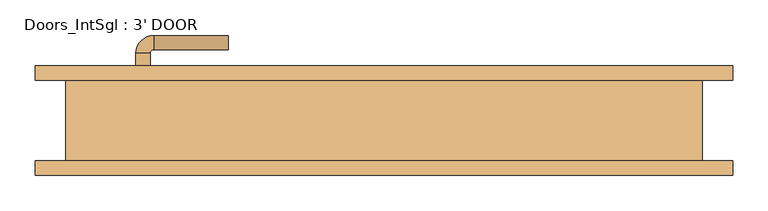
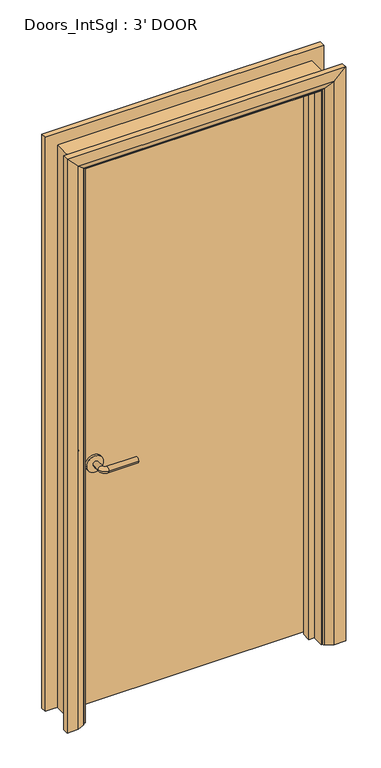
"""IFC4 building model written with IfcOpenShell, lengths in millimetres: door geometry, Doors_IntSgl : 3' DOOR."""

from ifc_helpers import new_model, si_unit, point, frame, frame_2d, origin, place, context, project, spatial, polyline, circle_curve, ellipse_curve, trimmed, segment, composite_curve, outline, extrude, faceted_brep, source, transform, mapped, element, save
from ifc_brep_helpers import plane_surface, cylinder_surface, revolved_surface, advanced_brep


def doors_intsgl_3_door_77e94e6e(model_context):
    return source(origin(), model_context, "Body", "SolidModel", [
        advanced_brep(
        [(-350.2, 11.15, 900.0), (-330.2, 11.15, 900.0), (-330.2, -18.85, 900.0), (-350.2, -18.85, 900.0), (-325.2, -23.85, 900.0), (-325.2, -43.85, 900.0), (-220.2, -43.85, 900.0), (-220.2, -23.85, 900.0)],
        [
            (0, 1, circle_curve(frame((-340.2, 11.15, 900.0), z_axis=(0.0, 1.0, 0.0), x_axis=(1.0, 0.0, 0.0)), 10.0)),
            (1, 0, circle_curve(frame((-340.2, 11.15, 900.0), z_axis=(0.0, 1.0, 0.0), x_axis=(1.0, 0.0, 0.0)), 10.0)),
            (1, 2),
            (2, 3, circle_curve(frame((-340.2, -18.85, 900.0), z_axis=(0.0, 1.0, 0.0), x_axis=(1.0, 0.0, 0.0)), 10.0)),
            (3, 0),
            (3, 2, circle_curve(frame((-340.2, -18.85, 900.0), z_axis=(0.0, 1.0, 0.0), x_axis=(1.0, 0.0, 0.0)), 10.0)),
            (4, 5, circle_curve(frame((-325.2, -33.85, 900.0), z_axis=(-1.0, 0.0, 0.0), x_axis=(0.0, 1.0, 0.0)), 10.0)),
            (5, 3, circle_curve(frame((-325.2, -18.85, 900.0), z_axis=(0.0, 0.0, -1.0), x_axis=(-1.0, 0.0, 0.0)), 25.0)),
            (2, 4, circle_curve(frame((-325.2, -18.85, 900.0), z_axis=(0.0, 0.0, 1.0), x_axis=(-1.0, 0.0, 0.0)), 5.0)),
            (5, 4, circle_curve(frame((-325.2, -33.85, 900.0), z_axis=(-1.0, 0.0, 0.0), x_axis=(0.0, 1.0, 0.0)), 10.0)),
            (6, 7, circle_curve(frame((-220.2, -33.85, 900.0), z_axis=(1.0, 0.0, 0.0), x_axis=(0.0, 1.0, 0.0)), 10.0)),
            (7, 6, circle_curve(frame((-220.2, -33.85, 900.0), z_axis=(1.0, 0.0, 0.0), x_axis=(0.0, 1.0, 0.0)), 10.0)),
            (4, 7),
            (6, 5),
        ],
        [
            plane_surface(frame((-340.2, 11.15, 900.0), z_axis=(0.0, 1.0, 0.0), x_axis=(0.0, 0.0, 1.0))),
            cylinder_surface(frame((-340.2, 11.15, 900.0), z_axis=(0.0, 1.0, 0.0), x_axis=(1.0, 0.0, 0.0)), 10.0),
            revolved_surface(trimmed(ellipse_curve(frame((-340.2, -18.85, 900.0), z_axis=(0.0, -1.0, 0.0), x_axis=(1.0, 0.0, 0.0)), 10.0, 10.0), [point((-350.2, -18.85, 900.0))], [point((-330.2, -18.85, 900.0))], True, "CARTESIAN"), (-325.2, -18.85, 900.0), (0.0, 0.0, -1.0)),
            revolved_surface(trimmed(ellipse_curve(frame((-340.2, -18.85, 900.0), z_axis=(0.0, -1.0, 0.0), x_axis=(1.0, 0.0, 0.0)), 10.0, 10.0), [point((-330.2, -18.85, 900.0))], [point((-350.2, -18.85, 900.0))], True, "CARTESIAN"), (-325.2, -18.85, 900.0), (0.0, 0.0, -1.0)),
            plane_surface(frame((-220.2, -33.85, 900.0), z_axis=(1.0, 0.0, 0.0), x_axis=(0.0, 0.0, 1.0))),
            cylinder_surface(frame((-325.2, -33.85, 900.0), z_axis=(-1.0, 0.0, 0.0), x_axis=(0.0, 1.0, 0.0)), 10.0),
        ],
        [
            (0, [[1, 2]]),
            (1, [[3, 4, 5, -2]]),
            (1, [[-5, 6, -3, -1]]),
            (2, [[7, 8, -4, 9]]),
            (3, [[10, -9, -6, -8]]),
            (4, [[11, 12]]),
            (5, [[13, -11, 14, -7]]),
            (5, [[-14, -12, -13, -10]]),
        ],
    ),
        extrude(outline(composite_curve([segment(trimmed(circle_curve(frame_2d((900.0, -342.7)), 30.0), [point((900.0, -372.7))], [point((900.0, -312.7))], False, "CARTESIAN"), True, "CONTINUOUS"), segment(trimmed(circle_curve(frame_2d((900.0, -342.7)), 30.0), [point((900.0, -312.7))], [point((900.0, -372.7))], False, "CARTESIAN"), True, "CONTINUOUS")], self_intersect=False)), frame((0.0, 11.15, 0.0), z_axis=(0.0, 1.0, 0.0), x_axis=(0.0, 0.0, 1.0)), (0.0, 0.0, 1.0), 8.0),
        advanced_brep(
        [(-350.2, 65.15, 900.0), (-330.2, 65.15, 900.0), (-350.2, 95.15, 900.0), (-330.2, 95.15, 900.0), (-325.2, 100.15, 900.0), (-325.2, 120.15, 900.0), (-220.2, 120.15, 900.0), (-220.2, 100.15, 900.0)],
        [
            (0, 1, circle_curve(frame((-340.2, 65.15, 900.0), z_axis=(0.0, -1.0, 0.0), x_axis=(1.0, 0.0, 0.0)), 10.0)),
            (1, 0, circle_curve(frame((-340.2, 65.15, 900.0), z_axis=(0.0, -1.0, 0.0), x_axis=(1.0, 0.0, 0.0)), 10.0)),
            (0, 2),
            (2, 3, circle_curve(frame((-340.2, 95.15, 900.0), z_axis=(0.0, -1.0, 0.0), x_axis=(1.0, 0.0, 0.0)), 10.0)),
            (3, 1),
            (3, 2, circle_curve(frame((-340.2, 95.15, 900.0), z_axis=(0.0, -1.0, 0.0), x_axis=(1.0, 0.0, 0.0)), 10.0)),
            (4, 3, circle_curve(frame((-325.2, 95.15, 900.0), z_axis=(0.0, 0.0, 1.0), x_axis=(-1.0, 0.0, 0.0)), 5.0)),
            (2, 5, circle_curve(frame((-325.2, 95.15, 900.0), z_axis=(0.0, 0.0, -1.0), x_axis=(-1.0, 0.0, 0.0)), 25.0)),
            (5, 4, circle_curve(frame((-325.2, 110.15, 900.0), z_axis=(-1.0, 0.0, 0.0), x_axis=(0.0, -1.0, 0.0)), 10.0)),
            (4, 5, circle_curve(frame((-325.2, 110.15, 900.0), z_axis=(-1.0, 0.0, 0.0), x_axis=(0.0, -1.0, 0.0)), 10.0)),
            (6, 7, circle_curve(frame((-220.2, 110.15, 900.0), z_axis=(1.0, 0.0, 0.0), x_axis=(0.0, -1.0, 0.0)), 10.0)),
            (7, 6, circle_curve(frame((-220.2, 110.15, 900.0), z_axis=(1.0, 0.0, 0.0), x_axis=(0.0, -1.0, 0.0)), 10.0)),
            (5, 6),
            (7, 4),
        ],
        [
            plane_surface(frame((-340.2, 65.15, 900.0), z_axis=(0.0, -1.0, 0.0), x_axis=(0.0, 0.0, 1.0))),
            cylinder_surface(frame((-340.2, 65.15, 900.0), z_axis=(0.0, -1.0, 0.0), x_axis=(1.0, 0.0, 0.0)), 10.0),
            revolved_surface(trimmed(ellipse_curve(frame((-340.2, 95.15, 900.0), z_axis=(0.0, -1.0, 0.0), x_axis=(1.0, 0.0, 0.0)), 10.0, 10.0), [point((-350.2, 95.15, 900.0))], [point((-330.2, 95.15, 900.0))], True, "CARTESIAN"), (-325.2, 95.15, 900.0), (0.0, 0.0, -1.0)),
            revolved_surface(trimmed(ellipse_curve(frame((-340.2, 95.15, 900.0), z_axis=(0.0, -1.0, 0.0), x_axis=(1.0, 0.0, 0.0)), 10.0, 10.0), [point((-330.2, 95.15, 900.0))], [point((-350.2, 95.15, 900.0))], True, "CARTESIAN"), (-325.2, 95.15, 900.0), (0.0, 0.0, -1.0)),
            plane_surface(frame((-220.2, 110.15, 900.0), z_axis=(1.0, 0.0, 0.0), x_axis=(0.0, 0.0, 1.0))),
            cylinder_surface(frame((-325.2, 110.15, 900.0), z_axis=(-1.0, 0.0, 0.0), x_axis=(0.0, -1.0, 0.0)), 10.0),
        ],
        [
            (0, [[1, 2]]),
            (1, [[-1, 3, 4, 5]]),
            (1, [[-2, -5, 6, -3]]),
            (2, [[7, -4, 8, 9]]),
            (3, [[-8, -6, -7, 10]]),
            (4, [[11, 12]]),
            (5, [[-9, 13, -12, 14]]),
            (5, [[-10, -14, -11, -13]]),
        ],
    ),
        extrude(outline(composite_curve([segment(trimmed(circle_curve(frame_2d((900.0, -342.7)), 30.0), [point((900.0, -372.7))], [point((900.0, -312.7))], False, "CARTESIAN"), True, "CONTINUOUS"), segment(trimmed(circle_curve(frame_2d((900.0, -342.7)), 30.0), [point((900.0, -312.7))], [point((900.0, -372.7))], False, "CARTESIAN"), True, "CONTINUOUS")], self_intersect=False)), frame((0.0, 57.15, 0.0), z_axis=(0.0, 1.0, 0.0), x_axis=(0.0, 0.0, 1.0)), (0.0, 0.0, 1.0), 8.0),
        extrude(outline(polyline([(415.2, 19.15), (-415.2, 19.15), (-415.2, 57.15), (415.2, 57.15), (415.2, 19.15)])), frame((0.0, 0.0, 8.0), z_axis=(0.0, 0.0, 1.0), x_axis=(1.0, 0.0, 0.0)), (0.0, 0.0, 1.0), 2060.0),
        advanced_brep(
        [(492.2, 77.15, 0.0), (492.2, 57.15, 0.0), (422.2, 57.15, 0.0), (426.2, 63.15, 0.0), (452.2, 77.15, 0.0), (492.2, 77.15, 2145.0), (492.2, 57.15, 2145.0), (-492.2, 57.15, 2145.0), (-492.2, 57.15, 0.0), (-422.2, 57.15, 0.0), (-422.2, 57.15, 2075.0), (422.2, 57.15, 2075.0), (426.2, 63.15, 2079.0), (452.2, 77.15, 2105.0), (-452.2, 77.15, 2105.0), (-452.2, 77.15, 0.0), (-492.2, 77.15, 0.0), (-492.2, 77.15, 2145.0), (-426.2, 63.15, 0.0), (-426.2, 63.15, 2079.0)],
        [
            (0, 1),
            (1, 2),
            (2, 3, circle_curve(frame((430.2, 56.15, 0.0), z_axis=(0.0, 0.0, -1.0), x_axis=(1.0, 0.0, 0.0)), 8.0622577)),
            (3, 4),
            (4, 0),
            (0, 5),
            (5, 6),
            (6, 1),
            (6, 7),
            (7, 8),
            (8, 9),
            (9, 10),
            (10, 11),
            (11, 2),
            (11, 12, ellipse_curve(frame((430.2, 56.15, 2083.0), z_axis=(0.7071067811865475, 0.0, -0.7071067811865475), x_axis=(-0.7071067811865474, 0.0, -0.7071067811865476)), 11.4017543, 8.0622577)),
            (12, 3),
            (12, 13),
            (13, 4),
            (13, 14),
            (14, 15),
            (15, 16),
            (16, 17),
            (17, 5),
            (7, 17),
            (16, 8),
            (15, 18),
            (18, 9, circle_curve(frame((-430.2, 56.15, 0.0), z_axis=(0.0, 0.0, -1.0), x_axis=(-1.0, 0.0, 0.0)), 8.0622577)),
            (19, 10, ellipse_curve(frame((-430.2, 56.15, 2083.0), z_axis=(-0.7071067811865475, 0.0, -0.7071067811865475), x_axis=(-0.7071067811865474, 0.0, 0.7071067811865476)), 11.4017543, 8.0622577)),
            (18, 19),
            (14, 19),
            (19, 12),
        ],
        [
            plane_surface(frame((422.2, 57.15, 0.0), z_axis=(0.0, 0.0, -1.0), x_axis=(0.0, -1.0, 0.0))),
            plane_surface(frame((492.2, 77.15, 0.0), z_axis=(1.0, 0.0, 0.0), x_axis=(0.0, 0.0, 1.0))),
            plane_surface(frame((492.2, 57.15, 0.0), z_axis=(0.0, -1.0, 0.0), x_axis=(0.0, 0.0, 1.0))),
            cylinder_surface(frame((430.2, 56.15, 0.0), z_axis=(0.0, 0.0, -1.0), x_axis=(1.0, 0.0, 0.0)), 8.0622577),
            plane_surface(frame((426.2, 63.15, 0.0), z_axis=(-0.4740998230350126, 0.880471099922178, 0.0), x_axis=(0.0, 0.0, 1.0))),
            plane_surface(frame((452.2, 77.15, 0.0), z_axis=(0.0, 1.0, 0.0), x_axis=(0.0, 0.0, 1.0))),
            plane_surface(frame((-492.2, 77.15, 2145.0), z_axis=(-1.0, 0.0, 0.0), x_axis=(0.0, 0.0, -1.0))),
            plane_surface(frame((-422.2, 57.15, 0.0), z_axis=(0.0, 0.0, -1.0), x_axis=(0.0, -1.0, 0.0))),
            cylinder_surface(frame((-430.2, 56.15, 2075.0), z_axis=(0.0, 0.0, 1.0), x_axis=(-1.0, 0.0, 0.0)), 8.0622577),
            plane_surface(frame((-426.2, 63.15, 2079.0), z_axis=(0.47409982303501824, 0.8804710999221749, 0.0), x_axis=(0.0, 0.0, -1.0))),
            plane_surface(frame((492.2, 77.15, 2145.0), z_axis=(0.0, 0.0, 1.0), x_axis=(-1.0, 0.0, 0.0))),
            cylinder_surface(frame((422.2, 56.15, 2083.0), z_axis=(1.0, 0.0, 0.0), x_axis=(0.0, 0.0, 1.0)), 8.0622577),
            plane_surface(frame((426.2, 63.15, 2079.0), z_axis=(0.0, 0.8804710999221764, -0.4740998230350154), x_axis=(-1.0, 0.0, 0.0))),
        ],
        [
            (0, [[1, 2, 3, 4, 5]]),
            (1, [[-1, 6, 7, 8]]),
            (2, [[-2, -8, 9, 10, 11, 12, 13, 14]]),
            (3, [[-3, -14, 15, 16]]),
            (4, [[-4, -16, 17, 18]]),
            (5, [[-5, -18, 19, 20, 21, 22, 23, -6]]),
            (6, [[24, -22, 25, -10]]),
            (7, [[-21, 26, 27, -11, -25]]),
            (8, [[28, -12, -27, 29]]),
            (9, [[30, -29, -26, -20]]),
            (10, [[-7, -23, -24, -9]]),
            (11, [[-15, -13, -28, 31]]),
            (12, [[-17, -31, -30, -19]]),
        ],
    ),
        extrude(outline(polyline([(0.0, -417.2), (0.0, -398.2), (2051.0, -398.2), (2051.0, 398.2), (0.0, 398.2), (0.0, 417.2), (2070.0, 417.2), (2070.0, -417.2), (0.0, -417.2)])), frame((0.0, -14.85, 0.0), z_axis=(0.0, 1.0, 0.0), x_axis=(0.0, 0.0, 1.0)), (0.0, 0.0, 1.0), 32.0),
        advanced_brep(
        [(-492.2, -77.15, 0.0), (-492.2, -57.15, 0.0), (-422.2, -57.15, 0.0), (-426.2, -63.15, 0.0), (-452.2, -77.15, 0.0), (-492.2, -77.15, 2145.0), (-492.2, -57.15, 2145.0), (-422.2, -57.15, 2075.0), (-426.2, -63.15, 2079.0), (-452.2, -77.15, 2105.0), (492.2, -77.15, 0.0), (452.2, -77.15, 0.0), (426.2, -63.15, 0.0), (422.2, -57.15, 0.0), (492.2, -57.15, 0.0), (492.2, -77.15, 2145.0), (452.2, -77.15, 2105.0), (426.2, -63.15, 2079.0), (422.2, -57.15, 2075.0), (492.2, -57.15, 2145.0)],
        [
            (0, 1),
            (1, 2),
            (2, 3, circle_curve(frame((-430.2, -56.15, 0.0), z_axis=(0.0, 0.0, -1.0), x_axis=(-1.0, 0.0, 0.0)), 8.0622577)),
            (3, 4),
            (4, 0),
            (0, 5),
            (5, 6),
            (6, 1),
            (6, 7),
            (7, 2),
            (7, 8, ellipse_curve(frame((-430.2, -56.15, 2083.0), z_axis=(-0.7071067811865475, 0.0, -0.7071067811865475), x_axis=(0.7071067811865474, 0.0, -0.7071067811865476)), 11.4017543, 8.0622577)),
            (8, 3),
            (8, 9),
            (9, 4),
            (9, 5),
            (10, 11),
            (11, 12),
            (12, 13, circle_curve(frame((430.2, -56.15, 0.0), z_axis=(0.0, 0.0, -1.0), x_axis=(1.0, 0.0, 0.0)), 8.0622577)),
            (13, 14),
            (14, 10),
            (15, 16),
            (16, 11),
            (10, 15),
            (16, 17),
            (17, 12),
            (17, 18, ellipse_curve(frame((430.2, -56.15, 2083.0), z_axis=(0.7071067811865475, 0.0, -0.7071067811865475), x_axis=(0.7071067811865474, 0.0, 0.7071067811865476)), 11.4017543, 8.0622577)),
            (18, 13),
            (18, 19),
            (19, 14),
            (19, 15),
            (5, 15),
            (19, 6),
            (18, 7),
            (17, 8),
            (16, 9),
        ],
        [
            plane_surface(frame((-422.2, -129.9510989, 0.0), z_axis=(0.0, 0.0, -1.0), x_axis=(1.0, 0.0, 0.0))),
            plane_surface(frame((-492.2, -77.15, 0.0), z_axis=(-1.0, 0.0, 0.0), x_axis=(0.0, 0.0, 1.0))),
            plane_surface(frame((-492.2, -57.15, 0.0), z_axis=(0.0, 1.0, 0.0), x_axis=(0.0, 0.0, 1.0))),
            cylinder_surface(frame((-430.2, -56.15, 0.0), z_axis=(0.0, 0.0, -1.0), x_axis=(-1.0, 0.0, 0.0)), 8.0622577),
            plane_surface(frame((-426.2, -63.15, 0.0), z_axis=(0.4740998230350183, -0.8804710999221749, 0.0), x_axis=(0.0, 0.0, 1.0))),
            plane_surface(frame((-452.2, -77.15, 0.0), z_axis=(0.0, -1.0, 0.0), x_axis=(0.0, 0.0, 1.0))),
            plane_surface(frame((422.2, -129.9510989, 0.0), z_axis=(0.0, 0.0, -1.0), x_axis=(-1.0, 0.0, 0.0))),
            plane_surface(frame((452.2, -77.15, 2105.0), z_axis=(0.0, -1.0, 0.0), x_axis=(0.0, 0.0, -1.0))),
            plane_surface(frame((426.2, -63.15, 2079.0), z_axis=(-0.4740998230350183, -0.8804710999221749, 0.0), x_axis=(0.0, 0.0, -1.0))),
            cylinder_surface(frame((430.2, -56.15, 2075.0), z_axis=(0.0, 0.0, 1.0), x_axis=(1.0, 0.0, 0.0)), 8.0622577),
            plane_surface(frame((492.2, -57.15, 2145.0), z_axis=(0.0, 1.0, 0.0), x_axis=(0.0, 0.0, -1.0))),
            plane_surface(frame((492.2, -77.15, 2145.0), z_axis=(1.0, 0.0, 0.0), x_axis=(0.0, 0.0, -1.0))),
            plane_surface(frame((-492.2, -77.15, 2145.0), z_axis=(0.0, 0.0, 1.0), x_axis=(1.0, 0.0, 0.0))),
            plane_surface(frame((-492.2, -57.15, 2145.0), z_axis=(0.0, 1.0, 0.0), x_axis=(1.0, 0.0, 0.0))),
            cylinder_surface(frame((-422.2, -56.15, 2083.0), z_axis=(-1.0, 0.0, 0.0), x_axis=(0.0, 0.0, 1.0)), 8.0622577),
            plane_surface(frame((-426.2, -63.15, 2079.0), z_axis=(0.0, -0.8804710999221749, -0.4740998230350183), x_axis=(1.0, 0.0, 0.0))),
            plane_surface(frame((-452.2, -77.15, 2105.0), z_axis=(0.0, -1.0, 0.0), x_axis=(1.0, 0.0, 0.0))),
        ],
        [
            (0, [[1, 2, 3, 4, 5]]),
            (1, [[-1, 6, 7, 8]]),
            (2, [[-2, -8, 9, 10]]),
            (3, [[-3, -10, 11, 12]]),
            (4, [[-4, -12, 13, 14]]),
            (5, [[-5, -14, 15, -6]]),
            (6, [[16, 17, 18, 19, 20]]),
            (7, [[21, 22, -16, 23]]),
            (8, [[24, 25, -17, -22]]),
            (9, [[26, 27, -18, -25]]),
            (10, [[28, 29, -19, -27]]),
            (11, [[30, -23, -20, -29]]),
            (12, [[-7, 31, -30, 32]]),
            (13, [[-9, -32, -28, 33]]),
            (14, [[-11, -33, -26, 34]]),
            (15, [[-13, -34, -24, 35]]),
            (16, [[-15, -35, -21, -31]]),
        ],
    ),
        faceted_brep([(-417.2, 57.15, 0.0), (-417.2, -57.15, 0.0), (-449.2, -57.15, 0.0), (-449.2, 57.15, 0.0), (-417.2, 57.15, 2070.0), (-417.2, -57.15, 2070.0), (-449.2, -57.15, 2102.0), (-449.2, 57.15, 2102.0), (417.2, 57.15, 0.0), (449.2, 57.15, 0.0), (449.2, -57.15, 0.0), (417.2, -57.15, 0.0), (417.2, 57.15, 2070.0), (449.2, 57.15, 2102.0), (449.2, -57.15, 2102.0), (417.2, -57.15, 2070.0)], [[[0, 1, 2, 3]], [[1, 0, 4, 5]], [[2, 1, 5, 6]], [[3, 2, 6, 7]], [[0, 3, 7, 4]], [[8, 9, 10, 11]], [[12, 13, 9, 8]], [[13, 14, 10, 9]], [[14, 15, 11, 10]], [[15, 12, 8, 11]], [[5, 4, 12, 15]], [[6, 5, 15, 14]], [[7, 6, 14, 13]], [[4, 7, 13, 12]]]),
    ])


if __name__ == "__main__":
    model = new_model("IFC4")
    model_context = context("Model", 3, world=origin())
    ifc_project = project(units=[si_unit("LENGTHUNIT", "METRE", prefix="MILLI")], contexts=[model_context])
    site = spatial("IfcSite", under=ifc_project)
    building = spatial("IfcBuilding", under=site)
    placement = place(None, origin())
    doors_intsgl_3_door_shape = doors_intsgl_3_door_77e94e6e(model_context)
    element("IfcDoor", 1, ObjectType="Doors_IntSgl : 3' DOOR", at=placement, inside=building, context=model_context, shape_type="MappedRepresentation", body=[
        mapped(doors_intsgl_3_door_shape, transform((0.0, 0.0, 0.0), x_axis=(1.0, 0.0, 0.0), y_axis=(0.0, 1.0, 0.0), z_axis=(0.0, 0.0, 1.0))),
    ])
    save(model, "model.ifc")

# Revit data of these elements
# Type "Doors_IntSgl : 3' DOOR"
#   Type Mark = "46"
#   Type Comments = "Internal Single"
#   Operation = "SingleSwingRight"
#   Manufacturer = "Revit"
#   Keynote = "L20"
#   Description = "Internal Single Door"
#   Analytic Construction = "Metal"
#   UnderCut = 0.026247 ft
#   Tolerance = 0.006562 ft
#   Thickness = 0.124672 ft
#   Thermal Resistance (R) = 0.270117 (m²·K)/W
#   Structural Tolerance = 0.026247 ft
#   StopDepth = 0.104987 ft
#   Stop Thickness = 0.062336 ft
#   Rough Width = 3.0 ft
#   Rough Height = 6.922572 ft
#   Height to Top Lock Rail = 3.28084 ft
#   Heat Transfer Coefficient (U) = 3.7021 W/(m²·K)
#   Handle Z Distance = 2.952756 ft
#   Handle X Distance = 0.246063 ft
#   Frame Thickness = 0.104987 ft
#   Door Panel Width = 2.724409 ft
#   Door Panel Thickness = 0.124672 ft
#   Door Panel Offset = 0.0 ft
#   Height = 6.922572 ft
#   Width = 3.0 ft
#   Door Panel Height = 6.75853 ft
#   Architrave Setback = 0.016404 ft
#   Vis - Ironmongery = yes
#   Material Ironmongery = Door - Handle
#   Material Frame = Door - Frame/Mullion (1)
#   Material Door = Door - Panel
#   Material Architrave = Door - Architrave
#   Visual Light Transmittance = 0
#   Solar Heat Gain Coefficient = 0
#   Function = (empty or 0)
#   Wall Closure = (empty or 0)
# Element 1 (IfcDoor, "Doors_IntSgl : 3' DOOR")
#   Materials on its faces: "Door - Architrave", "Door - Handle", "Door - Frame/Mullion (1)", "Door - Panel"
# Materials
#   "Door - Handle": colour RGB 0 0 0, transparency 0, Keynote = "P21", Cost = 0
#   "Door - Frame/Mullion (1)": class "Wood", colour RGB 212 179 113, transparency 0, Keynote = "L20", Cost = 0
#   "Door - Panel": class "Wood", colour RGB 210 159 95, transparency 0, Keynote = "L20", Cost = 0
#   "Door - Architrave": class "Wood", colour RGB 154 90 5, transparency 0, Keynote = "P20", Cost = 0
